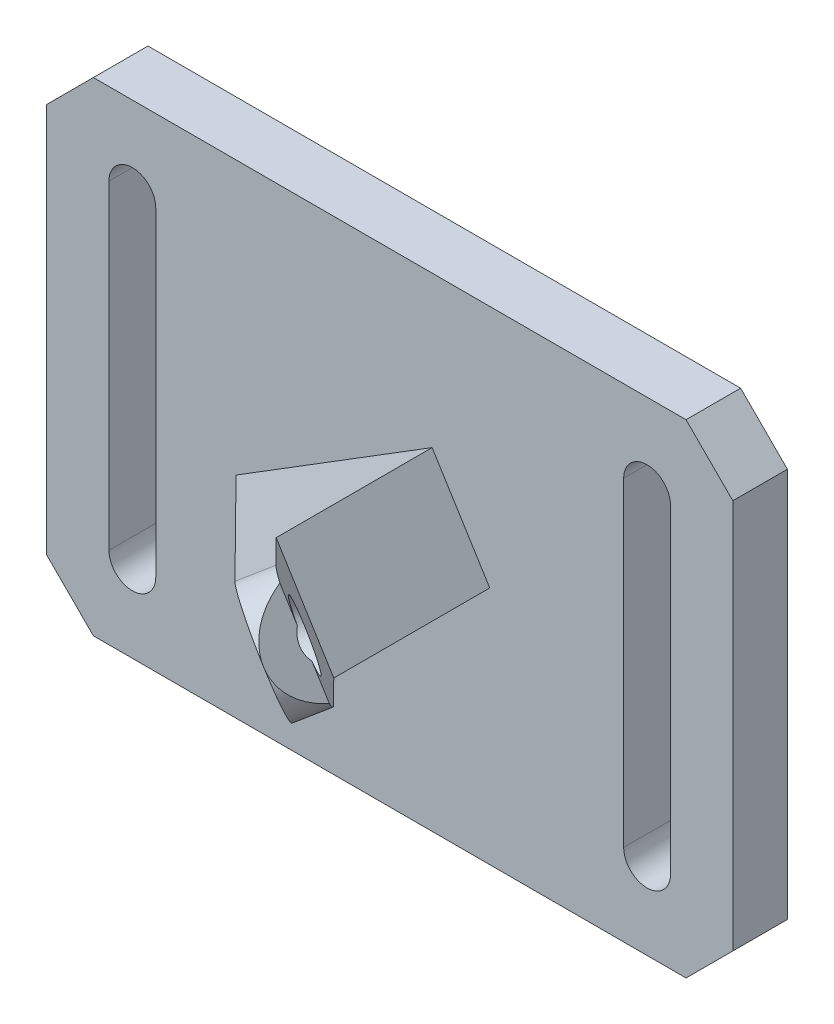
ISO-10303-21;
HEADER;
FILE_DESCRIPTION(('STEP AP214'),'2;1');
FILE_NAME('part.step','',(''),(''),'','','');
FILE_SCHEMA(('AUTOMOTIVE_DESIGN { 1 0 10303 214 1 1 1 1 }'));
ENDSEC;
DATA;
#1=APPLICATION_CONTEXT('core data for automotive mechanical design processes');
#2=APPLICATION_PROTOCOL_DEFINITION('international standard','automotive_design',2000,#1);
#3=PRODUCT_CONTEXT('',#1,'mechanical');
#4=PRODUCT('Part','Part','',(#3));
#5=PRODUCT_RELATED_PRODUCT_CATEGORY('part','',(#4));
#6=PRODUCT_DEFINITION_FORMATION('','',#4);
#7=PRODUCT_DEFINITION_CONTEXT('part definition',#1,'design');
#8=PRODUCT_DEFINITION('design','',#6,#7);
#9=PRODUCT_DEFINITION_SHAPE('','',#8);
#10=(LENGTH_UNIT() NAMED_UNIT(*) SI_UNIT(.MILLI.,.METRE.));
#11=(NAMED_UNIT(*) PLANE_ANGLE_UNIT() SI_UNIT($,.RADIAN.));
#12=(NAMED_UNIT(*) SI_UNIT($,.STERADIAN.) SOLID_ANGLE_UNIT());
#13=UNCERTAINTY_MEASURE_WITH_UNIT(LENGTH_MEASURE(1.E-05),#10,'distance_accuracy_value','');
#14=(GEOMETRIC_REPRESENTATION_CONTEXT(3) GLOBAL_UNCERTAINTY_ASSIGNED_CONTEXT((#13)) GLOBAL_UNIT_ASSIGNED_CONTEXT((#10,
#11,#12)) REPRESENTATION_CONTEXT('',''));
#15=CARTESIAN_POINT('',(0.,0.,0.));
#16=DIRECTION('',(0.,0.,1.));
#17=DIRECTION('',(1.,0.,0.));
#18=AXIS2_PLACEMENT_3D('',#15,#16,#17);
#19=CARTESIAN_POINT('',(15.7793177936232,18.0430146411911,50.));
#20=DIRECTION('',(-0.849441251034907,-0.527683201400473,0.));
#21=DIRECTION('',(0.527683201400473,-0.849441251034907,0.));
#22=AXIS2_PLACEMENT_3D('',#19,#20,#21);
#23=PLANE('',#22);
#24=CARTESIAN_POINT('',(19.4731002034265,12.0969258839468,31.8591294504759));
#25=DIRECTION('',(-0.849441251034907,-0.527683201400473,0.));
#26=DIRECTION('',(0.,0.,1.));
#27=AXIS2_PLACEMENT_3D('',#24,#25,#26);
#28=ELLIPSE('',#27,10.7844220546235,7.);
#29=CARTESIAN_POINT('',(19.4731002034265,12.0969258839468,42.6435515050994));
#30=VERTEX_POINT('',#29);
#31=CARTESIAN_POINT('',(16.3011338270231,17.2030180996204,37.3853502239355));
#32=VERTEX_POINT('',#31);
#33=EDGE_CURVE('E163',#30,#32,#28,.T.);
#34=ORIENTED_EDGE('',*,*,#33,.F.);
#35=CARTESIAN_POINT('',(19.4731002034265,12.0969258839468,31.8591294504759));
#36=DIRECTION('',(-0.849441251034907,-0.527683201400473,0.));
#37=DIRECTION('',(0.,0.,-1.));
#38=AXIS2_PLACEMENT_3D('',#35,#36,#37);
#39=ELLIPSE('',#38,10.7844220546235,7.);
#40=CARTESIAN_POINT('',(22.6450665798298,6.99083366827311,37.3853502239355));
#41=VERTEX_POINT('',#40);
#42=EDGE_CURVE('E316',#30,#41,#39,.F.);
#43=ORIENTED_EDGE('',*,*,#42,.T.);
#44=DIRECTION('',(0.527683201400473,-0.849441251034907,0.));
#45=VECTOR('',#44,1.);
#46=CARTESIAN_POINT('',(-6.673992723524,54.1873681565987,37.3853502239356));
#47=LINE('',#46,#45);
#48=CARTESIAN_POINT('',(20.4071961185791,10.5932592888229,37.3853502239355));
#49=VERTEX_POINT('',#48);
#50=EDGE_CURVE('E329',#49,#41,#47,.T.);
#51=ORIENTED_EDGE('',*,*,#50,.F.);
#52=CARTESIAN_POINT('',(19.4731002034265,12.0969258839468,31.8591294504759));
#53=DIRECTION('',(-0.849441251034907,-0.527683201400473,0.));
#54=DIRECTION('',(0.,0.,-1.));
#55=AXIS2_PLACEMENT_3D('',#52,#53,#54);
#56=ELLIPSE('',#55,6.16252688835631,4.00000000000001);
#57=CARTESIAN_POINT('',(18.5390042882738,13.6005924790706,37.3853502239355));
#58=VERTEX_POINT('',#57);
#59=EDGE_CURVE('E484',#58,#49,#56,.F.);
#60=ORIENTED_EDGE('',*,*,#59,.F.);
#61=EDGE_CURVE('E317',#32,#58,#47,.T.);
#62=ORIENTED_EDGE('',*,*,#61,.F.);
#63=EDGE_LOOP('',(#34,#43,#51,#60,#62));
#64=FACE_BOUND('',#63,.T.);
#65=ADVANCED_FACE('F146',(#64),#23,.F.);
#66=CARTESIAN_POINT('',(-35.8287649357497,36.0760702671858,13.3579138637895));
#67=DIRECTION('',(0.551359055415967,0.342510928364464,-0.760716409683481));
#68=DIRECTION('',(-0.80969153798108,0.,-0.586855700595839));
#69=AXIS2_PLACEMENT_3D('',#66,#67,#68);
#70=PLANE('',#69);
#71=CARTESIAN_POINT('',(14.9498129123562,9.2870049910092,38.0999607821276));
#72=DIRECTION('',(0.551359055415967,0.342510928364464,-0.760716409683481));
#73=DIRECTION('',(-0.80969153798108,0.,-0.586855700595839));
#74=AXIS2_PLACEMENT_3D('',#71,#72,#73);
#75=CIRCLE('',#74,4.00000000000001);
#76=CARTESIAN_POINT('',(11.7110467604319,9.2870049910092,35.7525379797442));
#77=VERTEX_POINT('',#76);
#78=EDGE_CURVE('E322',#77,#77,#75,.F.);
#79=ORIENTED_EDGE('',*,*,#78,.F.);
#80=EDGE_LOOP('',(#79));
#81=FACE_BOUND('',#80,.T.);
#82=CARTESIAN_POINT('',(14.9498129123562,9.28700499100919,38.0999607821276));
#83=DIRECTION('',(0.551359055415967,0.342510928364464,-0.760716409683481));
#84=DIRECTION('',(-0.80969153798108,0.,-0.586855700595839));
#85=AXIS2_PLACEMENT_3D('',#82,#83,#84);
#86=CIRCLE('',#85,7.);
#87=CARTESIAN_POINT('',(11.2560305025529,15.2330937482535,38.0999607821276));
#88=VERTEX_POINT('',#87);
#89=EDGE_CURVE('E303',#88,#30,#86,.T.);
#90=ORIENTED_EDGE('',*,*,#89,.F.);
#91=DIRECTION('',(0.646183898724319,0.401417270419653,0.649084388995972));
#92=VECTOR('',#91,1.);
#93=CARTESIAN_POINT('',(-1.66955850255724,7.20356118447297,25.1163533936458));
#94=LINE('',#93,#92);
#95=CARTESIAN_POINT('',(-19.7049573891052,-4.00024721474619,7.));
#96=VERTEX_POINT('',#95);
#97=EDGE_CURVE('E336',#96,#88,#94,.T.);
#98=ORIENTED_EDGE('',*,*,#97,.F.);
#99=DIRECTION('',(0.527683201400473,-0.849441251034907,0.));
#100=VECTOR('',#99,1.);
#101=CARTESIAN_POINT('',(-16.0111749793019,-9.94633597199054,7.));
#102=LINE('',#101,#100);
#103=CARTESIAN_POINT('',(-12.3173925694985,-15.8924247292349,7.));
#104=VERTEX_POINT('',#103);
#105=EDGE_CURVE('E353',#96,#104,#102,.T.);
#106=ORIENTED_EDGE('',*,*,#105,.T.);
#107=DIRECTION('',(-0.646183898724319,-0.401417270419652,-0.649084388995972));
#108=VECTOR('',#107,1.);
#109=CARTESIAN_POINT('',(5.71800631704939,-4.68861633001575,25.1163533936458));
#110=LINE('',#109,#108);
#111=CARTESIAN_POINT('',(18.6435953221596,3.34091623376481,38.0999607821276));
#112=VERTEX_POINT('',#111);
#113=EDGE_CURVE('E328',#112,#104,#110,.T.);
#114=ORIENTED_EDGE('',*,*,#113,.F.);
#115=CARTESIAN_POINT('',(14.9498129123562,9.2870049910092,38.0999607821276));
#116=DIRECTION('',(0.551359055415967,0.342510928364464,-0.760716409683481));
#117=DIRECTION('',(-0.80969153798108,0.,-0.586855700595839));
#118=AXIS2_PLACEMENT_3D('',#115,#116,#117);
#119=CIRCLE('',#118,7.);
#120=EDGE_CURVE('E323',#112,#30,#119,.F.);
#121=ORIENTED_EDGE('',*,*,#120,.T.);
#122=EDGE_LOOP('',(#90,#98,#106,#114,#121));
#123=FACE_BOUND('',#122,.T.);
#124=ADVANCED_FACE('F330',(#81,#123),#70,.F.);
#125=CARTESIAN_POINT('',(-33.6233287140859,37.4461139806436,10.3150482250555));
#126=DIRECTION('',(0.551359055415967,0.342510928364464,-0.760716409683481));
#127=DIRECTION('',(-0.80969153798108,0.,-0.586855700595839));
#128=AXIS2_PLACEMENT_3D('',#125,#126,#127);
#129=PLANE('',#128);
#130=DIRECTION('',(0.646183898724319,0.401417270419653,0.649084388995972));
#131=VECTOR('',#130,1.);
#132=CARTESIAN_POINT('',(0.535877719106626,8.57360489793083,22.0734877549119));
#133=LINE('',#132,#131);
#134=CARTESIAN_POINT('',(5.44037541403405,11.6203383144767,27.));
#135=VERTEX_POINT('',#134);
#136=CARTESIAN_POINT('',(13.4614667242168,16.6031374617114,35.0570951433936));
#137=VERTEX_POINT('',#136);
#138=EDGE_CURVE('E345',#135,#137,#133,.T.);
#139=ORIENTED_EDGE('',*,*,#138,.T.);
#140=CARTESIAN_POINT('',(17.1552491340201,10.6570487044671,35.0570951433936));
#141=DIRECTION('',(0.551359055415967,0.342510928364464,-0.760716409683481));
#142=DIRECTION('',(-0.80969153798108,0.,-0.586855700595839));
#143=AXIS2_PLACEMENT_3D('',#140,#141,#142);
#144=CIRCLE('',#143,7.);
#145=EDGE_CURVE('E319',#137,#32,#144,.T.);
#146=ORIENTED_EDGE('',*,*,#145,.T.);
#147=ORIENTED_EDGE('',*,*,#61,.T.);
#148=CARTESIAN_POINT('',(17.1552491340201,10.6570487044671,35.0570951433936));
#149=DIRECTION('',(0.551359055415967,0.342510928364464,-0.760716409683481));
#150=DIRECTION('',(-0.80969153798108,0.,-0.586855700595839));
#151=AXIS2_PLACEMENT_3D('',#148,#149,#150);
#152=CIRCLE('',#151,4.00000000000001);
#153=EDGE_CURVE('E479',#58,#49,#152,.F.);
#154=ORIENTED_EDGE('',*,*,#153,.T.);
#155=ORIENTED_EDGE('',*,*,#50,.T.);
#156=CARTESIAN_POINT('',(17.1552491340201,10.6570487044671,35.0570951433936));
#157=DIRECTION('',(0.551359055415967,0.342510928364464,-0.760716409683481));
#158=DIRECTION('',(-0.80969153798108,0.,-0.586855700595839));
#159=AXIS2_PLACEMENT_3D('',#156,#157,#158);
#160=CIRCLE('',#159,7.);
#161=CARTESIAN_POINT('',(20.8490315438235,4.71095994722267,35.0570951433936));
#162=VERTEX_POINT('',#161);
#163=EDGE_CURVE('E155',#162,#41,#160,.F.);
#164=ORIENTED_EDGE('',*,*,#163,.F.);
#165=DIRECTION('',(-0.646183898724319,-0.401417270419652,-0.649084388995972));
#166=VECTOR('',#165,1.);
#167=CARTESIAN_POINT('',(7.92344253871326,-3.3185726165579,22.0734877549119));
#168=LINE('',#167,#166);
#169=CARTESIAN_POINT('',(12.8279402336407,-0.271839200012069,27.));
#170=VERTEX_POINT('',#169);
#171=EDGE_CURVE('E478',#162,#170,#168,.T.);
#172=ORIENTED_EDGE('',*,*,#171,.T.);
#173=DIRECTION('',(0.527683201400473,-0.849441251034907,0.));
#174=VECTOR('',#173,1.);
#175=CARTESIAN_POINT('',(-17.0129351031131,47.7646918298843,27.));
#176=LINE('',#175,#174);
#177=EDGE_CURVE('E337',#135,#170,#176,.T.);
#178=ORIENTED_EDGE('',*,*,#177,.F.);
#179=EDGE_LOOP('',(#139,#146,#147,#154,#155,#164,#172,#178));
#180=FACE_BOUND('',#179,.T.);
#181=ADVANCED_FACE('F483',(#180),#129,.T.);
#182=CARTESIAN_POINT('',(-19.7049573891052,-4.00024721474619,50.));
#183=DIRECTION('',(0.527683201400473,-0.849441251034907,0.));
#184=DIRECTION('',(0.849441251034907,0.527683201400473,0.));
#185=AXIS2_PLACEMENT_3D('',#182,#183,#184);
#186=PLANE('',#185);
#187=DIRECTION('',(-0.551359055415967,-0.342510928364465,0.760716409683481));
#188=VECTOR('',#187,1.);
#189=CARTESIAN_POINT('',(18.4236982229605,19.6857358169916,28.2106474562423));
#190=LINE('',#189,#188);
#191=EDGE_CURVE('E12',#137,#88,#190,.T.);
#192=ORIENTED_EDGE('',*,*,#191,.F.);
#193=ORIENTED_EDGE('',*,*,#138,.F.);
#194=DIRECTION('',(0.,0.,1.));
#195=VECTOR('',#194,1.);
#196=CARTESIAN_POINT('',(5.44037541403405,11.6203383144767,50.));
#197=LINE('',#196,#195);
#198=CARTESIAN_POINT('',(5.44037541403405,11.6203383144767,7.));
#199=VERTEX_POINT('',#198);
#200=EDGE_CURVE('E347',#199,#135,#197,.T.);
#201=ORIENTED_EDGE('',*,*,#200,.F.);
#202=DIRECTION('',(-0.849441251034907,-0.527683201400473,0.));
#203=VECTOR('',#202,1.);
#204=CARTESIAN_POINT('',(-3.69378240980331,5.94608875724435,7.));
#205=LINE('',#204,#203);
#206=EDGE_CURVE('E351',#199,#96,#205,.T.);
#207=ORIENTED_EDGE('',*,*,#206,.T.);
#208=ORIENTED_EDGE('',*,*,#97,.T.);
#209=EDGE_LOOP('',(#192,#193,#201,#207,#208));
#210=FACE_BOUND('',#209,.T.);
#211=ADVANCED_FACE('F492',(#210),#186,.F.);
#212=CARTESIAN_POINT('',(-12.3173925694985,-15.8924247292349,50.));
#213=DIRECTION('',(-0.527683201400472,0.849441251034908,0.));
#214=DIRECTION('',(-0.849441251034908,-0.527683201400472,0.));
#215=AXIS2_PLACEMENT_3D('',#212,#213,#214);
#216=PLANE('',#215);
#217=DIRECTION('',(0.551359055415967,0.342510928364465,-0.760716409683481));
#218=VECTOR('',#217,1.);
#219=CARTESIAN_POINT('',(-8.79072823009513,-13.701618094151,75.9514115015162));
#220=LINE('',#219,#218);
#221=EDGE_CURVE('E175',#112,#162,#220,.T.);
#222=ORIENTED_EDGE('',*,*,#221,.F.);
#223=ORIENTED_EDGE('',*,*,#113,.T.);
#224=DIRECTION('',(0.849441251034908,0.527683201400472,0.));
#225=VECTOR('',#224,1.);
#226=CARTESIAN_POINT('',(3.69378240980332,-5.94608875724437,7.));
#227=LINE('',#226,#225);
#228=CARTESIAN_POINT('',(12.8279402336407,-0.271839200012065,7.));
#229=VERTEX_POINT('',#228);
#230=EDGE_CURVE('E346',#104,#229,#227,.T.);
#231=ORIENTED_EDGE('',*,*,#230,.T.);
#232=DIRECTION('',(0.,0.,-1.));
#233=VECTOR('',#232,1.);
#234=CARTESIAN_POINT('',(12.8279402336407,-0.271839200012076,50.));
#235=LINE('',#234,#233);
#236=EDGE_CURVE('E476',#170,#229,#235,.T.);
#237=ORIENTED_EDGE('',*,*,#236,.F.);
#238=ORIENTED_EDGE('',*,*,#171,.F.);
#239=EDGE_LOOP('',(#222,#223,#231,#237,#238));
#240=FACE_BOUND('',#239,.T.);
#241=ADVANCED_FACE('F501',(#240),#216,.F.);
#242=CARTESIAN_POINT('',(0.,0.,7.));
#243=DIRECTION('',(0.,0.,-1.));
#244=DIRECTION('',(-1.,0.,0.));
#245=AXIS2_PLACEMENT_3D('',#242,#243,#244);
#246=PLANE('',#245);
#247=ORIENTED_EDGE('',*,*,#206,.F.);
#248=DIRECTION('',(0.527683201400473,-0.849441251034907,0.));
#249=VECTOR('',#248,1.);
#250=CARTESIAN_POINT('',(-17.0129351031131,47.7646918298843,7.));
#251=LINE('',#250,#249);
#252=EDGE_CURVE('E333',#199,#229,#251,.T.);
#253=ORIENTED_EDGE('',*,*,#252,.T.);
#254=ORIENTED_EDGE('',*,*,#230,.F.);
#255=ORIENTED_EDGE('',*,*,#105,.F.);
#256=EDGE_LOOP('',(#247,#253,#254,#255));
#257=FACE_BOUND('',#256,.T.);
#258=CARTESIAN_POINT('',(33.,-20.5,7.));
#259=DIRECTION('',(0.,0.,1.));
#260=DIRECTION('',(1.,0.,0.));
#261=AXIS2_PLACEMENT_3D('',#258,#259,#260);
#262=CIRCLE('',#261,3.);
#263=CARTESIAN_POINT('',(30.,-20.5,7.));
#264=VERTEX_POINT('',#263);
#265=CARTESIAN_POINT('',(36.,-20.5,7.));
#266=VERTEX_POINT('',#265);
#267=EDGE_CURVE('E362',#264,#266,#262,.T.);
#268=ORIENTED_EDGE('',*,*,#267,.F.);
#269=DIRECTION('',(0.,-1.,0.));
#270=VECTOR('',#269,1.);
#271=CARTESIAN_POINT('',(30.,20.5,7.));
#272=LINE('',#271,#270);
#273=CARTESIAN_POINT('',(30.,20.5,7.));
#274=VERTEX_POINT('',#273);
#275=EDGE_CURVE('E358',#274,#264,#272,.T.);
#276=ORIENTED_EDGE('',*,*,#275,.F.);
#277=CARTESIAN_POINT('',(33.,20.5,7.));
#278=DIRECTION('',(0.,0.,1.));
#279=DIRECTION('',(1.,0.,0.));
#280=AXIS2_PLACEMENT_3D('',#277,#278,#279);
#281=CIRCLE('',#280,2.99999999999999);
#282=CARTESIAN_POINT('',(36.,20.5,7.));
#283=VERTEX_POINT('',#282);
#284=EDGE_CURVE('E356',#283,#274,#281,.T.);
#285=ORIENTED_EDGE('',*,*,#284,.F.);
#286=DIRECTION('',(0.,1.,0.));
#287=VECTOR('',#286,1.);
#288=CARTESIAN_POINT('',(36.,20.5,7.));
#289=LINE('',#288,#287);
#290=EDGE_CURVE('E364',#266,#283,#289,.T.);
#291=ORIENTED_EDGE('',*,*,#290,.F.);
#292=EDGE_LOOP('',(#268,#276,#285,#291));
#293=FACE_BOUND('',#292,.T.);
#294=CARTESIAN_POINT('',(-33.,20.5,7.));
#295=DIRECTION('',(0.,0.,1.));
#296=DIRECTION('',(1.,0.,0.));
#297=AXIS2_PLACEMENT_3D('',#294,#295,#296);
#298=CIRCLE('',#297,3.);
#299=CARTESIAN_POINT('',(-30.,20.5,7.));
#300=VERTEX_POINT('',#299);
#301=CARTESIAN_POINT('',(-36.,20.5,7.));
#302=VERTEX_POINT('',#301);
#303=EDGE_CURVE('E389',#300,#302,#298,.T.);
#304=ORIENTED_EDGE('',*,*,#303,.F.);
#305=DIRECTION('',(0.,1.,0.));
#306=VECTOR('',#305,1.);
#307=CARTESIAN_POINT('',(-30.,20.5,7.));
#308=LINE('',#307,#306);
#309=CARTESIAN_POINT('',(-30.,-20.5,7.));
#310=VERTEX_POINT('',#309);
#311=EDGE_CURVE('E399',#310,#300,#308,.T.);
#312=ORIENTED_EDGE('',*,*,#311,.F.);
#313=CARTESIAN_POINT('',(-33.,-20.5,7.));
#314=DIRECTION('',(0.,0.,1.));
#315=DIRECTION('',(1.,0.,0.));
#316=AXIS2_PLACEMENT_3D('',#313,#314,#315);
#317=CIRCLE('',#316,3.);
#318=CARTESIAN_POINT('',(-36.,-20.5,7.));
#319=VERTEX_POINT('',#318);
#320=EDGE_CURVE('E391',#319,#310,#317,.T.);
#321=ORIENTED_EDGE('',*,*,#320,.F.);
#322=DIRECTION('',(0.,-1.,0.));
#323=VECTOR('',#322,1.);
#324=CARTESIAN_POINT('',(-36.,20.5,7.));
#325=LINE('',#324,#323);
#326=EDGE_CURVE('E388',#302,#319,#325,.T.);
#327=ORIENTED_EDGE('',*,*,#326,.F.);
#328=EDGE_LOOP('',(#304,#312,#321,#327));
#329=FACE_BOUND('',#328,.T.);
#330=DIRECTION('',(1.,0.,0.));
#331=VECTOR('',#330,1.);
#332=CARTESIAN_POINT('',(-38.,-31.,7.));
#333=LINE('',#332,#331);
#334=CARTESIAN_POINT('',(-38.,-31.,7.));
#335=VERTEX_POINT('',#334);
#336=CARTESIAN_POINT('',(38.,-31.,7.));
#337=VERTEX_POINT('',#336);
#338=EDGE_CURVE('E428',#335,#337,#333,.T.);
#339=ORIENTED_EDGE('',*,*,#338,.T.);
#340=DIRECTION('',(0.707106781186549,0.707106781186546,0.));
#341=VECTOR('',#340,1.);
#342=CARTESIAN_POINT('',(38.,-31.,7.));
#343=LINE('',#342,#341);
#344=CARTESIAN_POINT('',(44.,-25.,7.));
#345=VERTEX_POINT('',#344);
#346=EDGE_CURVE('E429',#337,#345,#343,.T.);
#347=ORIENTED_EDGE('',*,*,#346,.T.);
#348=DIRECTION('',(0.,1.,0.));
#349=VECTOR('',#348,1.);
#350=CARTESIAN_POINT('',(44.,25.,7.));
#351=LINE('',#350,#349);
#352=CARTESIAN_POINT('',(44.,25.,7.));
#353=VERTEX_POINT('',#352);
#354=EDGE_CURVE('E435',#345,#353,#351,.T.);
#355=ORIENTED_EDGE('',*,*,#354,.T.);
#356=DIRECTION('',(-0.707106781186549,0.707106781186546,0.));
#357=VECTOR('',#356,1.);
#358=CARTESIAN_POINT('',(38.,31.,7.));
#359=LINE('',#358,#357);
#360=CARTESIAN_POINT('',(38.,31.,7.));
#361=VERTEX_POINT('',#360);
#362=EDGE_CURVE('E432',#353,#361,#359,.T.);
#363=ORIENTED_EDGE('',*,*,#362,.T.);
#364=DIRECTION('',(-1.,0.,0.));
#365=VECTOR('',#364,1.);
#366=CARTESIAN_POINT('',(-38.,31.,7.));
#367=LINE('',#366,#365);
#368=CARTESIAN_POINT('',(-38.,31.,7.));
#369=VERTEX_POINT('',#368);
#370=EDGE_CURVE('E420',#361,#369,#367,.T.);
#371=ORIENTED_EDGE('',*,*,#370,.T.);
#372=DIRECTION('',(-0.707106781186549,-0.707106781186546,0.));
#373=VECTOR('',#372,1.);
#374=CARTESIAN_POINT('',(-44.,25.,7.));
#375=LINE('',#374,#373);
#376=CARTESIAN_POINT('',(-44.,25.,7.));
#377=VERTEX_POINT('',#376);
#378=EDGE_CURVE('E423',#369,#377,#375,.T.);
#379=ORIENTED_EDGE('',*,*,#378,.T.);
#380=DIRECTION('',(0.,-1.,0.));
#381=VECTOR('',#380,1.);
#382=CARTESIAN_POINT('',(-44.,25.,7.));
#383=LINE('',#382,#381);
#384=CARTESIAN_POINT('',(-44.,-25.,7.));
#385=VERTEX_POINT('',#384);
#386=EDGE_CURVE('E424',#377,#385,#383,.T.);
#387=ORIENTED_EDGE('',*,*,#386,.T.);
#388=DIRECTION('',(0.707106781186548,-0.707106781186547,0.));
#389=VECTOR('',#388,1.);
#390=CARTESIAN_POINT('',(-44.,-25.,7.));
#391=LINE('',#390,#389);
#392=EDGE_CURVE('E426',#385,#335,#391,.T.);
#393=ORIENTED_EDGE('',*,*,#392,.T.);
#394=EDGE_LOOP('',(#339,#347,#355,#363,#371,#379,#387,#393));
#395=FACE_BOUND('',#394,.T.);
#396=ADVANCED_FACE('F496',(#257,#293,#329,#395),#246,.F.);
#397=CARTESIAN_POINT('',(0.,0.,0.));
#398=DIRECTION('',(0.,0.,-1.));
#399=DIRECTION('',(-1.,0.,0.));
#400=AXIS2_PLACEMENT_3D('',#397,#398,#399);
#401=PLANE('',#400);
#402=DIRECTION('',(-1.,0.,0.));
#403=VECTOR('',#402,1.);
#404=CARTESIAN_POINT('',(-38.,31.,0.));
#405=LINE('',#404,#403);
#406=CARTESIAN_POINT('',(38.,31.,0.));
#407=VERTEX_POINT('',#406);
#408=CARTESIAN_POINT('',(-38.,31.,0.));
#409=VERTEX_POINT('',#408);
#410=EDGE_CURVE('E416',#407,#409,#405,.T.);
#411=ORIENTED_EDGE('',*,*,#410,.F.);
#412=DIRECTION('',(-0.707106781186549,0.707106781186546,0.));
#413=VECTOR('',#412,1.);
#414=CARTESIAN_POINT('',(38.,31.,0.));
#415=LINE('',#414,#413);
#416=CARTESIAN_POINT('',(44.,25.,0.));
#417=VERTEX_POINT('',#416);
#418=EDGE_CURVE('E425',#417,#407,#415,.T.);
#419=ORIENTED_EDGE('',*,*,#418,.F.);
#420=DIRECTION('',(0.,1.,0.));
#421=VECTOR('',#420,1.);
#422=CARTESIAN_POINT('',(44.,25.,0.));
#423=LINE('',#422,#421);
#424=CARTESIAN_POINT('',(44.,-25.,0.));
#425=VERTEX_POINT('',#424);
#426=EDGE_CURVE('E447',#425,#417,#423,.T.);
#427=ORIENTED_EDGE('',*,*,#426,.F.);
#428=DIRECTION('',(0.707106781186549,0.707106781186546,0.));
#429=VECTOR('',#428,1.);
#430=CARTESIAN_POINT('',(38.,-31.,0.));
#431=LINE('',#430,#429);
#432=CARTESIAN_POINT('',(38.,-31.,0.));
#433=VERTEX_POINT('',#432);
#434=EDGE_CURVE('E450',#433,#425,#431,.T.);
#435=ORIENTED_EDGE('',*,*,#434,.F.);
#436=DIRECTION('',(1.,0.,0.));
#437=VECTOR('',#436,1.);
#438=CARTESIAN_POINT('',(-38.,-31.,0.));
#439=LINE('',#438,#437);
#440=CARTESIAN_POINT('',(-38.,-31.,0.));
#441=VERTEX_POINT('',#440);
#442=EDGE_CURVE('E443',#441,#433,#439,.T.);
#443=ORIENTED_EDGE('',*,*,#442,.F.);
#444=DIRECTION('',(0.707106781186548,-0.707106781186547,0.));
#445=VECTOR('',#444,1.);
#446=CARTESIAN_POINT('',(-44.,-25.,0.));
#447=LINE('',#446,#445);
#448=CARTESIAN_POINT('',(-44.,-25.,0.));
#449=VERTEX_POINT('',#448);
#450=EDGE_CURVE('E444',#449,#441,#447,.T.);
#451=ORIENTED_EDGE('',*,*,#450,.F.);
#452=DIRECTION('',(0.,-1.,0.));
#453=VECTOR('',#452,1.);
#454=CARTESIAN_POINT('',(-44.,25.,0.));
#455=LINE('',#454,#453);
#456=CARTESIAN_POINT('',(-44.,25.,0.));
#457=VERTEX_POINT('',#456);
#458=EDGE_CURVE('E442',#457,#449,#455,.T.);
#459=ORIENTED_EDGE('',*,*,#458,.F.);
#460=DIRECTION('',(-0.707106781186549,-0.707106781186546,0.));
#461=VECTOR('',#460,1.);
#462=CARTESIAN_POINT('',(-44.,25.,0.));
#463=LINE('',#462,#461);
#464=EDGE_CURVE('E438',#409,#457,#463,.T.);
#465=ORIENTED_EDGE('',*,*,#464,.F.);
#466=EDGE_LOOP('',(#411,#419,#427,#435,#443,#451,#459,#465));
#467=FACE_BOUND('',#466,.T.);
#468=DIRECTION('',(0.,1.,0.));
#469=VECTOR('',#468,1.);
#470=CARTESIAN_POINT('',(-30.,20.5,0.));
#471=LINE('',#470,#469);
#472=CARTESIAN_POINT('',(-30.,-20.5,0.));
#473=VERTEX_POINT('',#472);
#474=CARTESIAN_POINT('',(-30.,20.5,0.));
#475=VERTEX_POINT('',#474);
#476=EDGE_CURVE('E393',#473,#475,#471,.T.);
#477=ORIENTED_EDGE('',*,*,#476,.T.);
#478=CARTESIAN_POINT('',(-33.,20.5,0.));
#479=DIRECTION('',(0.,0.,1.));
#480=DIRECTION('',(1.,0.,0.));
#481=AXIS2_PLACEMENT_3D('',#478,#479,#480);
#482=CIRCLE('',#481,3.);
#483=CARTESIAN_POINT('',(-36.,20.5,0.));
#484=VERTEX_POINT('',#483);
#485=EDGE_CURVE('E390',#475,#484,#482,.T.);
#486=ORIENTED_EDGE('',*,*,#485,.T.);
#487=DIRECTION('',(0.,-1.,0.));
#488=VECTOR('',#487,1.);
#489=CARTESIAN_POINT('',(-36.,20.5,0.));
#490=LINE('',#489,#488);
#491=CARTESIAN_POINT('',(-36.,-20.5,0.));
#492=VERTEX_POINT('',#491);
#493=EDGE_CURVE('E402',#484,#492,#490,.T.);
#494=ORIENTED_EDGE('',*,*,#493,.T.);
#495=CARTESIAN_POINT('',(-33.,-20.5,0.));
#496=DIRECTION('',(0.,0.,1.));
#497=DIRECTION('',(1.,0.,0.));
#498=AXIS2_PLACEMENT_3D('',#495,#496,#497);
#499=CIRCLE('',#498,3.);
#500=EDGE_CURVE('E404',#492,#473,#499,.T.);
#501=ORIENTED_EDGE('',*,*,#500,.T.);
#502=EDGE_LOOP('',(#477,#486,#494,#501));
#503=FACE_BOUND('',#502,.T.);
#504=DIRECTION('',(0.,1.,0.));
#505=VECTOR('',#504,1.);
#506=CARTESIAN_POINT('',(36.,20.5,0.));
#507=LINE('',#506,#505);
#508=CARTESIAN_POINT('',(36.,-20.5,0.));
#509=VERTEX_POINT('',#508);
#510=CARTESIAN_POINT('',(36.,20.5,0.));
#511=VERTEX_POINT('',#510);
#512=EDGE_CURVE('E357',#509,#511,#507,.T.);
#513=ORIENTED_EDGE('',*,*,#512,.T.);
#514=CARTESIAN_POINT('',(33.,20.5,0.));
#515=DIRECTION('',(0.,0.,1.));
#516=DIRECTION('',(1.,0.,0.));
#517=AXIS2_PLACEMENT_3D('',#514,#515,#516);
#518=CIRCLE('',#517,2.99999999999999);
#519=CARTESIAN_POINT('',(30.,20.5,0.));
#520=VERTEX_POINT('',#519);
#521=EDGE_CURVE('E359',#511,#520,#518,.T.);
#522=ORIENTED_EDGE('',*,*,#521,.T.);
#523=DIRECTION('',(0.,-1.,0.));
#524=VECTOR('',#523,1.);
#525=CARTESIAN_POINT('',(30.,20.5,0.));
#526=LINE('',#525,#524);
#527=CARTESIAN_POINT('',(30.,-20.5,0.));
#528=VERTEX_POINT('',#527);
#529=EDGE_CURVE('E367',#520,#528,#526,.T.);
#530=ORIENTED_EDGE('',*,*,#529,.T.);
#531=CARTESIAN_POINT('',(33.,-20.5,0.));
#532=DIRECTION('',(0.,0.,1.));
#533=DIRECTION('',(1.,0.,0.));
#534=AXIS2_PLACEMENT_3D('',#531,#532,#533);
#535=CIRCLE('',#534,3.);
#536=EDGE_CURVE('E373',#528,#509,#535,.T.);
#537=ORIENTED_EDGE('',*,*,#536,.T.);
#538=EDGE_LOOP('',(#513,#522,#530,#537));
#539=FACE_BOUND('',#538,.T.);
#540=ADVANCED_FACE('F561',(#467,#503,#539),#401,.T.);
#541=CARTESIAN_POINT('',(-38.,31.,7.));
#542=DIRECTION('',(0.,-1.,0.));
#543=DIRECTION('',(0.,0.,-1.));
#544=AXIS2_PLACEMENT_3D('',#541,#542,#543);
#545=PLANE('',#544);
#546=ORIENTED_EDGE('',*,*,#410,.T.);
#547=DIRECTION('',(0.,0.,-1.));
#548=VECTOR('',#547,1.);
#549=CARTESIAN_POINT('',(-38.,31.,7.));
#550=LINE('',#549,#548);
#551=EDGE_CURVE('E472',#369,#409,#550,.T.);
#552=ORIENTED_EDGE('',*,*,#551,.F.);
#553=ORIENTED_EDGE('',*,*,#370,.F.);
#554=DIRECTION('',(0.,0.,-1.));
#555=VECTOR('',#554,1.);
#556=CARTESIAN_POINT('',(38.,31.,7.));
#557=LINE('',#556,#555);
#558=EDGE_CURVE('E436',#361,#407,#557,.T.);
#559=ORIENTED_EDGE('',*,*,#558,.T.);
#560=EDGE_LOOP('',(#546,#552,#553,#559));
#561=FACE_BOUND('',#560,.T.);
#562=ADVANCED_FACE('F147',(#561),#545,.F.);
#563=CARTESIAN_POINT('',(-44.,25.,7.));
#564=DIRECTION('',(0.707106781186546,-0.707106781186549,0.));
#565=DIRECTION('',(0.707106781186549,0.707106781186546,0.));
#566=AXIS2_PLACEMENT_3D('',#563,#564,#565);
#567=PLANE('',#566);
#568=ORIENTED_EDGE('',*,*,#464,.T.);
#569=DIRECTION('',(0.,0.,-1.));
#570=VECTOR('',#569,1.);
#571=CARTESIAN_POINT('',(-44.,25.,7.));
#572=LINE('',#571,#570);
#573=EDGE_CURVE('E468',#377,#457,#572,.T.);
#574=ORIENTED_EDGE('',*,*,#573,.F.);
#575=ORIENTED_EDGE('',*,*,#378,.F.);
#576=ORIENTED_EDGE('',*,*,#551,.T.);
#577=EDGE_LOOP('',(#568,#574,#575,#576));
#578=FACE_BOUND('',#577,.T.);
#579=ADVANCED_FACE('F590',(#578),#567,.F.);
#580=CARTESIAN_POINT('',(-44.,25.,7.));
#581=DIRECTION('',(1.,0.,0.));
#582=DIRECTION('',(0.,0.,-1.));
#583=AXIS2_PLACEMENT_3D('',#580,#581,#582);
#584=PLANE('',#583);
#585=ORIENTED_EDGE('',*,*,#458,.T.);
#586=DIRECTION('',(0.,0.,-1.));
#587=VECTOR('',#586,1.);
#588=CARTESIAN_POINT('',(-44.,-25.,7.));
#589=LINE('',#588,#587);
#590=EDGE_CURVE('E469',#385,#449,#589,.T.);
#591=ORIENTED_EDGE('',*,*,#590,.F.);
#592=ORIENTED_EDGE('',*,*,#386,.F.);
#593=ORIENTED_EDGE('',*,*,#573,.T.);
#594=EDGE_LOOP('',(#585,#591,#592,#593));
#595=FACE_BOUND('',#594,.T.);
#596=ADVANCED_FACE('F585',(#595),#584,.F.);
#597=CARTESIAN_POINT('',(-44.,-25.,7.));
#598=DIRECTION('',(0.707106781186547,0.707106781186548,0.));
#599=DIRECTION('',(-0.707106781186548,0.707106781186547,0.));
#600=AXIS2_PLACEMENT_3D('',#597,#598,#599);
#601=PLANE('',#600);
#602=ORIENTED_EDGE('',*,*,#450,.T.);
#603=DIRECTION('',(0.,0.,-1.));
#604=VECTOR('',#603,1.);
#605=CARTESIAN_POINT('',(-38.,-31.,7.));
#606=LINE('',#605,#604);
#607=EDGE_CURVE('E461',#335,#441,#606,.T.);
#608=ORIENTED_EDGE('',*,*,#607,.F.);
#609=ORIENTED_EDGE('',*,*,#392,.F.);
#610=ORIENTED_EDGE('',*,*,#590,.T.);
#611=EDGE_LOOP('',(#602,#608,#609,#610));
#612=FACE_BOUND('',#611,.T.);
#613=ADVANCED_FACE('F577',(#612),#601,.F.);
#614=CARTESIAN_POINT('',(-38.,-31.,7.));
#615=DIRECTION('',(0.,1.,0.));
#616=DIRECTION('',(-1.,0.,0.));
#617=AXIS2_PLACEMENT_3D('',#614,#615,#616);
#618=PLANE('',#617);
#619=ORIENTED_EDGE('',*,*,#442,.T.);
#620=DIRECTION('',(0.,0.,-1.));
#621=VECTOR('',#620,1.);
#622=CARTESIAN_POINT('',(38.,-31.,7.));
#623=LINE('',#622,#621);
#624=EDGE_CURVE('E458',#337,#433,#623,.T.);
#625=ORIENTED_EDGE('',*,*,#624,.F.);
#626=ORIENTED_EDGE('',*,*,#338,.F.);
#627=ORIENTED_EDGE('',*,*,#607,.T.);
#628=EDGE_LOOP('',(#619,#625,#626,#627));
#629=FACE_BOUND('',#628,.T.);
#630=ADVANCED_FACE('F579',(#629),#618,.F.);
#631=CARTESIAN_POINT('',(38.,-31.,7.));
#632=DIRECTION('',(-0.707106781186546,0.707106781186549,0.));
#633=DIRECTION('',(-0.707106781186549,-0.707106781186546,0.));
#634=AXIS2_PLACEMENT_3D('',#631,#632,#633);
#635=PLANE('',#634);
#636=ORIENTED_EDGE('',*,*,#434,.T.);
#637=DIRECTION('',(0.,0.,-1.));
#638=VECTOR('',#637,1.);
#639=CARTESIAN_POINT('',(44.,-25.,7.));
#640=LINE('',#639,#638);
#641=EDGE_CURVE('E460',#345,#425,#640,.T.);
#642=ORIENTED_EDGE('',*,*,#641,.F.);
#643=ORIENTED_EDGE('',*,*,#346,.F.);
#644=ORIENTED_EDGE('',*,*,#624,.T.);
#645=EDGE_LOOP('',(#636,#642,#643,#644));
#646=FACE_BOUND('',#645,.T.);
#647=ADVANCED_FACE('F575',(#646),#635,.F.);
#648=CARTESIAN_POINT('',(44.,25.,7.));
#649=DIRECTION('',(-1.,0.,0.));
#650=DIRECTION('',(0.,-1.,0.));
#651=AXIS2_PLACEMENT_3D('',#648,#649,#650);
#652=PLANE('',#651);
#653=ORIENTED_EDGE('',*,*,#426,.T.);
#654=DIRECTION('',(0.,0.,-1.));
#655=VECTOR('',#654,1.);
#656=CARTESIAN_POINT('',(44.,25.,7.));
#657=LINE('',#656,#655);
#658=EDGE_CURVE('E453',#353,#417,#657,.T.);
#659=ORIENTED_EDGE('',*,*,#658,.F.);
#660=ORIENTED_EDGE('',*,*,#354,.F.);
#661=ORIENTED_EDGE('',*,*,#641,.T.);
#662=EDGE_LOOP('',(#653,#659,#660,#661));
#663=FACE_BOUND('',#662,.T.);
#664=ADVANCED_FACE('F566',(#663),#652,.F.);
#665=CARTESIAN_POINT('',(38.,31.,7.));
#666=DIRECTION('',(-0.707106781186546,-0.707106781186549,0.));
#667=DIRECTION('',(0.707106781186549,-0.707106781186546,0.));
#668=AXIS2_PLACEMENT_3D('',#665,#666,#667);
#669=PLANE('',#668);
#670=ORIENTED_EDGE('',*,*,#418,.T.);
#671=ORIENTED_EDGE('',*,*,#558,.F.);
#672=ORIENTED_EDGE('',*,*,#362,.F.);
#673=ORIENTED_EDGE('',*,*,#658,.T.);
#674=EDGE_LOOP('',(#670,#671,#672,#673));
#675=FACE_BOUND('',#674,.T.);
#676=ADVANCED_FACE('F556',(#675),#669,.F.);
#677=CARTESIAN_POINT('',(-33.,20.5,7.));
#678=DIRECTION('',(0.,0.,-1.));
#679=DIRECTION('',(-1.,0.,0.));
#680=AXIS2_PLACEMENT_3D('',#677,#678,#679);
#681=CYLINDRICAL_SURFACE('',#680,3.);
#682=ORIENTED_EDGE('',*,*,#485,.F.);
#683=DIRECTION('',(0.,0.,-1.));
#684=VECTOR('',#683,1.);
#685=CARTESIAN_POINT('',(-30.,20.5,7.));
#686=LINE('',#685,#684);
#687=EDGE_CURVE('E400',#300,#475,#686,.T.);
#688=ORIENTED_EDGE('',*,*,#687,.F.);
#689=ORIENTED_EDGE('',*,*,#303,.T.);
#690=DIRECTION('',(0.,0.,-1.));
#691=VECTOR('',#690,1.);
#692=CARTESIAN_POINT('',(-36.,20.5,7.));
#693=LINE('',#692,#691);
#694=EDGE_CURVE('E412',#302,#484,#693,.T.);
#695=ORIENTED_EDGE('',*,*,#694,.T.);
#696=EDGE_LOOP('',(#682,#688,#689,#695));
#697=FACE_BOUND('',#696,.T.);
#698=ADVANCED_FACE('F551',(#697),#681,.F.);
#699=CARTESIAN_POINT('',(-36.,20.5,7.));
#700=DIRECTION('',(1.,0.,0.));
#701=DIRECTION('',(0.,1.,0.));
#702=AXIS2_PLACEMENT_3D('',#699,#700,#701);
#703=PLANE('',#702);
#704=ORIENTED_EDGE('',*,*,#493,.F.);
#705=ORIENTED_EDGE('',*,*,#694,.F.);
#706=ORIENTED_EDGE('',*,*,#326,.T.);
#707=DIRECTION('',(0.,0.,-1.));
#708=VECTOR('',#707,1.);
#709=CARTESIAN_POINT('',(-36.,-20.5,7.));
#710=LINE('',#709,#708);
#711=EDGE_CURVE('E415',#319,#492,#710,.T.);
#712=ORIENTED_EDGE('',*,*,#711,.T.);
#713=EDGE_LOOP('',(#704,#705,#706,#712));
#714=FACE_BOUND('',#713,.T.);
#715=ADVANCED_FACE('F549',(#714),#703,.T.);
#716=CARTESIAN_POINT('',(-33.,-20.5,7.));
#717=DIRECTION('',(0.,0.,-1.));
#718=DIRECTION('',(-1.,0.,0.));
#719=AXIS2_PLACEMENT_3D('',#716,#717,#718);
#720=CYLINDRICAL_SURFACE('',#719,3.);
#721=ORIENTED_EDGE('',*,*,#500,.F.);
#722=ORIENTED_EDGE('',*,*,#711,.F.);
#723=ORIENTED_EDGE('',*,*,#320,.T.);
#724=DIRECTION('',(0.,0.,-1.));
#725=VECTOR('',#724,1.);
#726=CARTESIAN_POINT('',(-30.,-20.5,7.));
#727=LINE('',#726,#725);
#728=EDGE_CURVE('E414',#310,#473,#727,.T.);
#729=ORIENTED_EDGE('',*,*,#728,.T.);
#730=EDGE_LOOP('',(#721,#722,#723,#729));
#731=FACE_BOUND('',#730,.T.);
#732=ADVANCED_FACE('F546',(#731),#720,.F.);
#733=CARTESIAN_POINT('',(-30.,20.5,7.));
#734=DIRECTION('',(-1.,0.,0.));
#735=DIRECTION('',(0.,0.,1.));
#736=AXIS2_PLACEMENT_3D('',#733,#734,#735);
#737=PLANE('',#736);
#738=ORIENTED_EDGE('',*,*,#476,.F.);
#739=ORIENTED_EDGE('',*,*,#728,.F.);
#740=ORIENTED_EDGE('',*,*,#311,.T.);
#741=ORIENTED_EDGE('',*,*,#687,.T.);
#742=EDGE_LOOP('',(#738,#739,#740,#741));
#743=FACE_BOUND('',#742,.T.);
#744=ADVANCED_FACE('F545',(#743),#737,.T.);
#745=CARTESIAN_POINT('',(33.,20.5,7.));
#746=DIRECTION('',(0.,0.,-1.));
#747=DIRECTION('',(-1.,0.,0.));
#748=AXIS2_PLACEMENT_3D('',#745,#746,#747);
#749=CYLINDRICAL_SURFACE('',#748,2.99999999999999);
#750=ORIENTED_EDGE('',*,*,#521,.F.);
#751=DIRECTION('',(0.,0.,-1.));
#752=VECTOR('',#751,1.);
#753=CARTESIAN_POINT('',(36.,20.5,7.));
#754=LINE('',#753,#752);
#755=EDGE_CURVE('E370',#283,#511,#754,.T.);
#756=ORIENTED_EDGE('',*,*,#755,.F.);
#757=ORIENTED_EDGE('',*,*,#284,.T.);
#758=DIRECTION('',(0.,0.,-1.));
#759=VECTOR('',#758,1.);
#760=CARTESIAN_POINT('',(30.,20.5,7.));
#761=LINE('',#760,#759);
#762=EDGE_CURVE('E383',#274,#520,#761,.T.);
#763=ORIENTED_EDGE('',*,*,#762,.T.);
#764=EDGE_LOOP('',(#750,#756,#757,#763));
#765=FACE_BOUND('',#764,.T.);
#766=ADVANCED_FACE('F538',(#765),#749,.F.);
#767=CARTESIAN_POINT('',(30.,20.5,7.));
#768=DIRECTION('',(1.,0.,0.));
#769=DIRECTION('',(0.,1.,0.));
#770=AXIS2_PLACEMENT_3D('',#767,#768,#769);
#771=PLANE('',#770);
#772=ORIENTED_EDGE('',*,*,#529,.F.);
#773=ORIENTED_EDGE('',*,*,#762,.F.);
#774=ORIENTED_EDGE('',*,*,#275,.T.);
#775=DIRECTION('',(0.,0.,-1.));
#776=VECTOR('',#775,1.);
#777=CARTESIAN_POINT('',(30.,-20.5,7.));
#778=LINE('',#777,#776);
#779=EDGE_CURVE('E385',#264,#528,#778,.T.);
#780=ORIENTED_EDGE('',*,*,#779,.T.);
#781=EDGE_LOOP('',(#772,#773,#774,#780));
#782=FACE_BOUND('',#781,.T.);
#783=ADVANCED_FACE('F534',(#782),#771,.T.);
#784=CARTESIAN_POINT('',(33.,-20.5,7.));
#785=DIRECTION('',(0.,0.,-1.));
#786=DIRECTION('',(-1.,0.,0.));
#787=AXIS2_PLACEMENT_3D('',#784,#785,#786);
#788=CYLINDRICAL_SURFACE('',#787,3.);
#789=ORIENTED_EDGE('',*,*,#536,.F.);
#790=ORIENTED_EDGE('',*,*,#779,.F.);
#791=ORIENTED_EDGE('',*,*,#267,.T.);
#792=DIRECTION('',(0.,0.,-1.));
#793=VECTOR('',#792,1.);
#794=CARTESIAN_POINT('',(36.,-20.5,7.));
#795=LINE('',#794,#793);
#796=EDGE_CURVE('E379',#266,#509,#795,.T.);
#797=ORIENTED_EDGE('',*,*,#796,.T.);
#798=EDGE_LOOP('',(#789,#790,#791,#797));
#799=FACE_BOUND('',#798,.T.);
#800=ADVANCED_FACE('F520',(#799),#788,.F.);
#801=CARTESIAN_POINT('',(36.,20.5,7.));
#802=DIRECTION('',(-1.,0.,0.));
#803=DIRECTION('',(0.,-1.,0.));
#804=AXIS2_PLACEMENT_3D('',#801,#802,#803);
#805=PLANE('',#804);
#806=ORIENTED_EDGE('',*,*,#512,.F.);
#807=ORIENTED_EDGE('',*,*,#796,.F.);
#808=ORIENTED_EDGE('',*,*,#290,.T.);
#809=ORIENTED_EDGE('',*,*,#755,.T.);
#810=EDGE_LOOP('',(#806,#807,#808,#809));
#811=FACE_BOUND('',#810,.T.);
#812=ADVANCED_FACE('F508',(#811),#805,.T.);
#813=CARTESIAN_POINT('',(-17.0129351031131,47.7646918298843,0.));
#814=DIRECTION('',(0.849441251034907,0.527683201400473,0.));
#815=DIRECTION('',(-0.527683201400473,0.849441251034907,0.));
#816=AXIS2_PLACEMENT_3D('',#813,#814,#815);
#817=PLANE('',#816);
#818=ORIENTED_EDGE('',*,*,#200,.T.);
#819=ORIENTED_EDGE('',*,*,#177,.T.);
#820=ORIENTED_EDGE('',*,*,#236,.T.);
#821=ORIENTED_EDGE('',*,*,#252,.F.);
#822=EDGE_LOOP('',(#818,#819,#820,#821));
#823=FACE_BOUND('',#822,.T.);
#824=ADVANCED_FACE('F509',(#823),#817,.T.);
#825=CARTESIAN_POINT('',(-12.4845106398985,-7.7555293369066,75.9514115015162));
#826=DIRECTION('',(0.551359055415967,0.342510928364465,-0.760716409683481));
#827=DIRECTION('',(-0.80969153798108,0.,-0.586855700595839));
#828=AXIS2_PLACEMENT_3D('',#825,#826,#827);
#829=CYLINDRICAL_SURFACE('',#828,4.00000000000001);
#830=ORIENTED_EDGE('',*,*,#59,.T.);
#831=ORIENTED_EDGE('',*,*,#153,.F.);
#832=EDGE_LOOP('',(#830,#831));
#833=FACE_BOUND('',#832,.T.);
#834=ORIENTED_EDGE('',*,*,#78,.T.);
#835=EDGE_LOOP('',(#834));
#836=FACE_BOUND('',#835,.T.);
#837=ADVANCED_FACE('F510',(#833,#836),#829,.F.);
#838=CARTESIAN_POINT('',(-12.4845106398985,-7.7555293369066,75.9514115015162));
#839=DIRECTION('',(0.551359055415967,0.342510928364465,-0.760716409683481));
#840=DIRECTION('',(-0.80969153798108,0.,-0.586855700595839));
#841=AXIS2_PLACEMENT_3D('',#838,#839,#840);
#842=CYLINDRICAL_SURFACE('',#841,7.);
#843=ORIENTED_EDGE('',*,*,#221,.T.);
#844=ORIENTED_EDGE('',*,*,#163,.T.);
#845=ORIENTED_EDGE('',*,*,#42,.F.);
#846=ORIENTED_EDGE('',*,*,#120,.F.);
#847=EDGE_LOOP('',(#843,#844,#845,#846));
#848=FACE_BOUND('',#847,.T.);
#849=ADVANCED_FACE('F325',(#848),#842,.T.);
#850=CARTESIAN_POINT('',(22.1174806327638,13.7396470597472,28.2106474562423));
#851=DIRECTION('',(-0.551359055415967,-0.342510928364465,0.760716409683481));
#852=DIRECTION('',(0.80969153798108,0.,0.586855700595839));
#853=AXIS2_PLACEMENT_3D('',#850,#851,#852);
#854=CYLINDRICAL_SURFACE('',#853,7.);
#855=ORIENTED_EDGE('',*,*,#89,.T.);
#856=ORIENTED_EDGE('',*,*,#33,.T.);
#857=ORIENTED_EDGE('',*,*,#145,.F.);
#858=ORIENTED_EDGE('',*,*,#191,.T.);
#859=EDGE_LOOP('',(#855,#856,#857,#858));
#860=FACE_BOUND('',#859,.T.);
#861=ADVANCED_FACE('F302',(#860),#854,.T.);
#862=CLOSED_SHELL('',(#65,#124,#181,#211,#241,#396,#540,#562,#579,#596,#613,#630,#647,#664,#676,
#698,#715,#732,#744,#766,#783,#800,#812,#824,#837,#849,#861));
#863=MANIFOLD_SOLID_BREP('B2',#862);
#864=ADVANCED_BREP_SHAPE_REPRESENTATION('',(#18,#863),#14);
#865=SHAPE_DEFINITION_REPRESENTATION(#9,#864);
ENDSEC;
END-ISO-10303-21;
